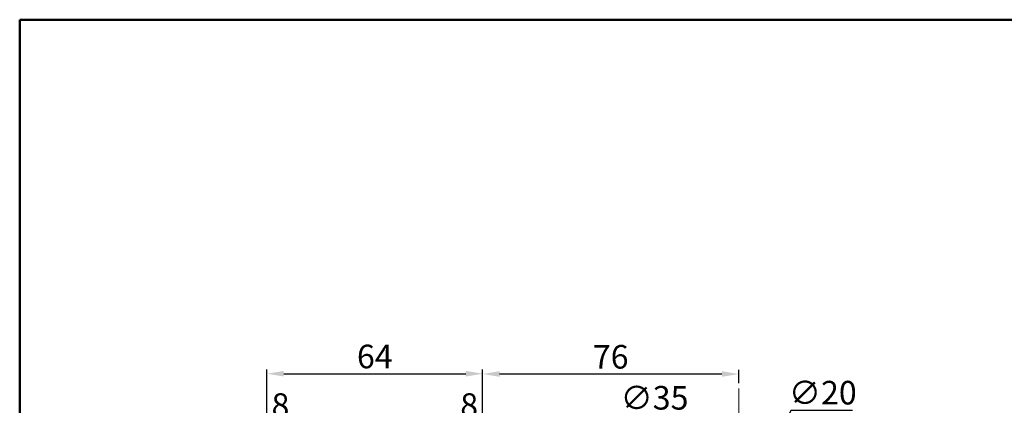
# Model space of a CAD drawing. Units: millimetres. Extents: x 434 to 1535, y -197 to 318.
# Tile 3 of 9: x 434 to 726, y 204 to 318. Entities that reach past the tile are written whole.
import ezdxf

# ---------------------------------------------------------------- set-up
doc = ezdxf.new("R2010")
doc.units = ezdxf.units.MM
doc.header["$LTSCALE"] = 0.4
doc.linetypes.add('CENTER2', pattern=[28.575, 19.05, -3.175, 3.175, -3.175])
for name, color, linetype, lineweight in [('M-CNTR', 1, 'CENTER2', 18), ('M-DIMS', 2, 'Continuous', 25), ('M-OUTL', 7, 'Continuous', 50)]:
    doc.layers.add(name, color=color, linetype=linetype, lineweight=lineweight)
doc.styles.get("Standard").update_dxf_attribs({"font": 'arial.ttf'})
doc.dimstyles.new('ISO-25', dxfattribs={"dimtxt": 7, "dimasz": 5, "dimexe": 1.25, "dimexo": 0.625, "dimtad": 1, "dimtoh": 1, "dimdec": 0, "dimtxsty": 'Standard', "dimcen": 2.5, "dimadec": 0, "dimazin": 0, "dimtfac": 1, "dimtdec": 0, "dimtmove": 0, "dimatfit": 3, "dimfxl": 1, "dimarcsym": 0})

# ---------------------------------------------------------------- blocks, each defined once
blk = doc.blocks.new('*U1')
at = {"layer": 'M-CNTR', "color": 0, "transparency": 16777216}
for p, q in [((0, 7), (0, 38.5)), ((-38.5, 0), (-7, 0)), ((7, 0), (73.2, 0)), ((0, -198.75), (0, -7))]:
    blk.add_line(p, q, dxfattribs=at)
at = {"layer": 'M-CNTR', "color": 0, "linetype": 'Continuous', "transparency": 16777216}
for p, q in [((0, -3.5), (0, 3.5)), ((-3.5, 0), (3.5, 0))]:
    blk.add_line(p, q, dxfattribs=at)
blk = doc.blocks.new('*D7')
at = {"layer": 'Defpoints', "color": 0, "ltscale": 0.4, "transparency": 16777216}
for p in [(515.58, 199.04), (507.58, 188.56), (515.58, 188.56)]:
    blk.add_point(p, dxfattribs=at)
at = {"layer": 'M-DIMS', "color": 0, "lineweight": -2, "ltscale": 0.4, "transparency": 16777216}
for p, q in [((502.58, 199.04), (497.58, 199.04)), ((507.58, 189.19), (507.58, 200.29)), ((507.58, 199.04), (515.58, 199.04)), ((515.58, 189.19), (515.58, 200.29)), ((520.58, 199.04), (525.58, 199.04))]:
    blk.add_line(p, q, dxfattribs=at)
at = {"layer": 'M-DIMS', "color": 0, "ltscale": 0.4, "transparency": 16777216}
for points in [[(502.58, 199.87), (502.58, 198.21), (507.58, 199.04)], [(520.58, 199.87), (520.58, 198.21), (515.58, 199.04)]]:
    blk.add_solid(points, dxfattribs=at)
at = {"layer": 'M-DIMS', "color": 0, "ltscale": 0.4, "transparency": 16777216, "insert": (511.58, 203.24), "char_height": 7, "attachment_point": 5}
blk.add_mtext('8', dxfattribs=at)
blk = doc.blocks.new('*D11')
at = {"layer": 'Defpoints', "color": 0, "ltscale": 0.4, "transparency": 16777216}
for p in [(571.58, 213.45), (507.58, 188.56), (571.58, 185.87)]:
    blk.add_point(p, dxfattribs=at)
at = {"layer": 'M-DIMS', "color": 0, "lineweight": -2, "ltscale": 0.4, "transparency": 16777216}
for p, q in [((507.58, 189.19), (507.58, 214.7)), ((512.58, 213.45), (566.58, 213.45)), ((571.58, 186.49), (571.58, 214.7))]:
    blk.add_line(p, q, dxfattribs=at)
at = {"layer": 'M-DIMS', "color": 0, "ltscale": 0.4, "transparency": 16777216}
for points in [[(512.58, 214.29), (512.58, 212.62), (507.58, 213.45)], [(566.58, 214.29), (566.58, 212.62), (571.58, 213.45)]]:
    blk.add_solid(points, dxfattribs=at)
at = {"layer": 'M-DIMS', "color": 0, "ltscale": 0.4, "transparency": 16777216, "insert": (539.58, 217.65), "char_height": 7, "attachment_point": 5}
blk.add_mtext('64', dxfattribs=at)
blk = doc.blocks.new('*D12')
at = {"layer": 'Defpoints', "color": 0, "ltscale": 0.4, "transparency": 16777216}
for p in [(571.58, 199.04), (563.58, 188.56), (571.58, 188.56)]:
    blk.add_point(p, dxfattribs=at)
at = {"layer": 'M-DIMS', "color": 0, "lineweight": -2, "ltscale": 0.4, "transparency": 16777216}
for p, q in [((558.58, 199.04), (553.58, 199.04)), ((563.58, 189.19), (563.58, 200.29)), ((563.58, 199.04), (571.58, 199.04)), ((571.58, 189.19), (571.58, 200.29)), ((576.58, 199.04), (581.58, 199.04))]:
    blk.add_line(p, q, dxfattribs=at)
at = {"layer": 'M-DIMS', "color": 0, "ltscale": 0.4, "transparency": 16777216}
for points in [[(558.58, 199.87), (558.58, 198.21), (563.58, 199.04)], [(576.58, 199.87), (576.58, 198.21), (571.58, 199.04)]]:
    blk.add_solid(points, dxfattribs=at)
at = {"layer": 'M-DIMS', "color": 0, "ltscale": 0.4, "transparency": 16777216, "insert": (567.58, 203.24), "char_height": 7, "attachment_point": 5}
blk.add_mtext('8', dxfattribs=at)
blk = doc.blocks.new('*D16')
at = {"layer": 'Defpoints', "color": 0, "ltscale": 0.4, "transparency": 16777216}
for p in [(571.58, 213.36), (571.58, 210.06), (647.58, 210.06)]:
    blk.add_point(p, dxfattribs=at)
at = {"layer": 'M-DIMS', "color": 0, "lineweight": -2, "ltscale": 0.4, "transparency": 16777216}
for p, q in [((571.58, 210.69), (571.58, 214.61)), ((642.58, 213.36), (576.58, 213.36)), ((647.58, 210.69), (647.58, 214.61))]:
    blk.add_line(p, q, dxfattribs=at)
at = {"layer": 'M-DIMS', "color": 0, "ltscale": 0.4, "transparency": 16777216}
for points in [[(576.58, 214.2), (576.58, 212.53), (571.58, 213.36)], [(642.58, 214.2), (642.58, 212.53), (647.58, 213.36)]]:
    blk.add_solid(points, dxfattribs=at)
at = {"layer": 'M-DIMS', "color": 0, "ltscale": 0.4, "transparency": 16777216, "insert": (609.58, 217.56), "char_height": 7, "attachment_point": 5}
blk.add_mtext('76', dxfattribs=at)
blk = doc.blocks.new('*D40')
at = {"layer": 'Defpoints', "color": 0, "ltscale": 0.4, "transparency": 16777216}
for p in [(639.42, 187.04), (655.74, 156.08)]:
    blk.add_point(p, dxfattribs=at)
at = {"layer": 'M-DIMS', "color": 0, "lineweight": -2, "ltscale": 0.4, "transparency": 16777216}
for p, q in [((613.74, 201), (632.06, 201)), ((632.06, 201), (637.08, 191.46)), ((655.74, 156.08), (639.42, 187.04)), ((658.07, 151.66), (660.4, 147.23))]:
    blk.add_line(p, q, dxfattribs=at)
at = {"layer": 'M-DIMS', "color": 0, "ltscale": 0.4, "transparency": 16777216}
for points in [[(637.82, 191.85), (636.35, 191.08), (639.42, 187.04)], [(658.8, 152.04), (657.33, 151.27), (655.74, 156.08)]]:
    blk.add_solid(points, dxfattribs=at)
at = {"layer": 'M-DIMS', "color": 0, "ltscale": 0.4, "transparency": 16777216, "insert": (622.58, 205.4), "char_height": 7, "attachment_point": 5}
blk.add_mtext('∅35', dxfattribs=at)
blk = doc.blocks.new('*D41')
at = {"layer": 'Defpoints', "color": 0, "ltscale": 0.4, "transparency": 16777216}
for p in [(652.05, 180.5), (643.1, 162.62)]:
    blk.add_point(p, dxfattribs=at)
at = {"layer": 'M-DIMS', "color": 0, "lineweight": -2, "ltscale": 0.4, "transparency": 16777216}
for p, q in [((663.07, 202.52), (654.29, 184.97)), ((681.32, 202.52), (663.07, 202.52)), ((643.1, 162.62), (652.05, 180.5)), ((640.86, 158.15), (638.62, 153.68))]:
    blk.add_line(p, q, dxfattribs=at)
at = {"layer": 'M-DIMS', "color": 0, "ltscale": 0.4, "transparency": 16777216}
for points in [[(653.54, 185.35), (655.03, 184.6), (652.05, 180.5)], [(640.12, 158.52), (641.61, 157.77), (643.1, 162.62)]]:
    blk.add_solid(points, dxfattribs=at)
at = {"layer": 'M-DIMS', "color": 0, "ltscale": 0.4, "transparency": 16777216, "insert": (672.51, 206.92), "char_height": 7, "attachment_point": 5}
blk.add_mtext('∅20', dxfattribs=at)

msp = doc.modelspace()

# ---------------------------------------------------------------- linework, layer by layer
at = {"layer": 'M-OUTL', "ltscale": 0.4}
msp.add_lwpolyline([(434.2, 318.45), (1535.47, 318.45), (1535.47, -197.48), (434.2, -197.48)], close=True, dxfattribs=at)

# ---------------------------------------------------------------- block references
at = {"layer": 'M-CNTR'}
msp.add_blockref('*U1', (647.58, 171.56), dxfattribs=at)

# ---------------------------------------------------------------- dimensions: what is measured, and where the dimension line sits
at = {"layer": 'M-DIMS', "ltscale": 0.4}
for base, p1, p2, picture, middle in [((571.58, 213.45), (507.58, 188.56), (571.58, 185.87), '*D11', (539.58, 217.65)), ((571.58, 213.36), (647.58, 210.06), (571.58, 210.06), '*D16', (609.58, 217.56)), ((515.58, 199.04), (507.58, 188.56), (515.58, 188.56), '*D7', (511.58, 203.24)), ((571.58, 199.04), (563.58, 188.56), (571.58, 188.56), '*D12', (567.58, 203.24))]:
    dim = msp.add_linear_dim(base=base, p1=p1, p2=p2, dimstyle='ISO-25', override={"dimclrd": 0, "dimclre": 0, "dimclrt": 0}, dxfattribs=at)
    dim.commit()
    dim.dimension.update_dxf_attribs({"geometry": picture, "text_midpoint": middle})
for p1, p2, picture, middle in [((643.1, 162.62), (652.05, 180.5), '*D41', (672.51, 202.52)), ((655.74, 156.08), (639.42, 187.04), '*D40', (622.58, 201))]:
    dim = msp.add_diameter_dim_2p(p1=p1, p2=p2, dimstyle='ISO-25', override={"dimclrd": 0, "dimclre": 0, "dimclrt": 0}, dxfattribs=at)
    dim.commit()
    dim.dimension.update_dxf_attribs({"geometry": picture, "text_midpoint": middle, "dimtype": 163})

doc.saveas('drawing.dxf')
